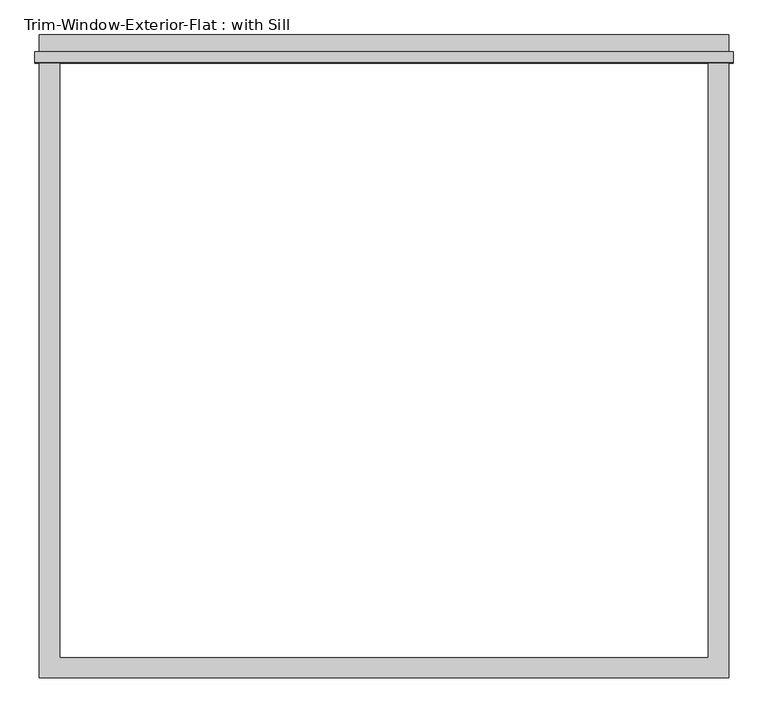
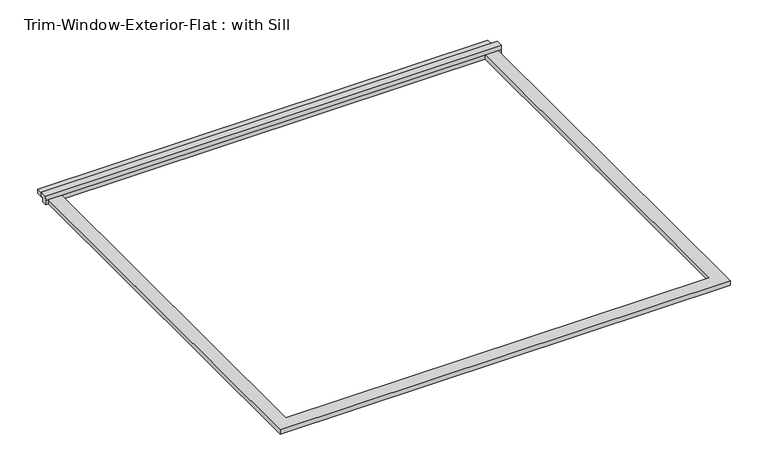
"""IFC4 building model written with IfcOpenShell, lengths in millimetres: proxy geometry, Trim-Window-Exterior-Flat : with Sill."""

from ifc_helpers import new_model, si_unit, frame, origin, origin_with_axes, place, context, project, spatial, polyline, outline, extrude, source, transform, mapped, element, save


def trim_window_exterior_flat_with_sill_2360300c(model_context):
    return source(origin(), model_context, "Body", "SweptSolid", [
        extrude(outline(polyline([(971.55, 1698.5823709), (-971.55, 1698.5823709), (-971.55, 1755.7323709), (971.55, 1755.7323709), (971.55, 1698.5823709)])), origin_with_axes(), (0.0, 0.0, 1.0), 19.05),
        extrude(outline(polyline([(1708.15, 38.1), (1708.15, 19.05), (1698.5823709, 19.05), (1698.5823709, 0.0), (1676.4, 0.0), (1676.4, 19.05), (1678.8580645, 38.1), (1708.15, 38.1)])), frame((-984.25, 0.0, 0.0), z_axis=(1.0, 0.0, 0.0), x_axis=(0.0, 1.0, 0.0)), (0.0, 0.0, 1.0), 1968.5),
        extrude(outline(polyline([(-971.55, -57.15), (-971.55, 1676.4), (-914.4, 1676.4), (-914.4, 0.0), (914.4, 0.0), (914.4, 1676.4), (971.55, 1676.4), (971.55, -57.15), (-971.55, -57.15)])), origin_with_axes(), (0.0, 0.0, 1.0), 19.05),
    ])


if __name__ == "__main__":
    model = new_model("IFC4")
    model_context = context("Model", 3, world=origin())
    ifc_project = project(units=[si_unit("LENGTHUNIT", "METRE", prefix="MILLI")], contexts=[model_context])
    site = spatial("IfcSite", under=ifc_project)
    building = spatial("IfcBuilding", under=site)
    placement = place(None, origin())
    trim_window_exterior_flat_with_sill_shape = trim_window_exterior_flat_with_sill_2360300c(model_context)
    element("IfcBuildingElementProxy", 1, Name="Trim-Window-Exterior-Flat : with Sill", ObjectType="Trim-Window-Exterior-Flat : with Sill", at=placement, inside=building, context=model_context, shape_type="MappedRepresentation", body=[
        mapped(trim_window_exterior_flat_with_sill_shape, transform((0.0, 0.0, 0.0), x_axis=(1.0, 0.0, 0.0), y_axis=(0.0, 1.0, 0.0), z_axis=(0.0, 0.0, 1.0))),
    ])
    save(model, "model.ifc")

# Revit data of these elements
# Type "Trim-Window-Exterior-Flat : with Sill"
#   Trim Width = 0' - 2 1/4"
#   Trim Thickness_Picture Frame = 0' - 1 1/4"
#   Trim Thickness_with Sill = 0' - 0 3/4"
#   Sill Thickness = 0' - 1 1/4"
#   Opening Width [instance default] = 2' - 0"
#   Opening Height [instance default] = 3' - 0"
#   Default Elevation = 4' - 0"
#   Sill = yes
#   Picture Frame = no
#   Trim Material [instance default] = none
# Element 1 (IfcBuildingElementProxy, "Trim-Window-Exterior-Flat : with Sill")
#   Opening Width = 6' - 0"
#   Opening Height = 5' - 6"
#   Trim Material = Clad - White
#   Materials on its faces: "Clad - White"
# Materials
#   "Clad - White": class "Wood", colour RGB 242 242 238, transparency 0, Cost = 0
